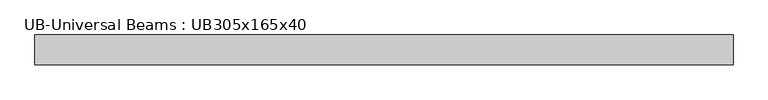
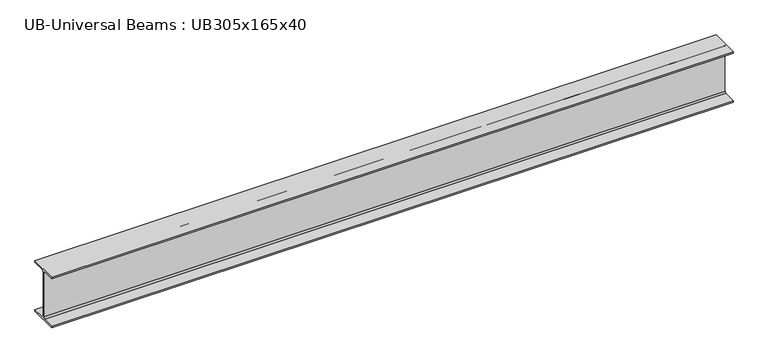
"""IFC4 building model written with IfcOpenShell, lengths in millimetres: beam geometry, UB-Universal Beams : UB305x165x40."""

from ifc_helpers import new_model, si_unit, point, frame, frame_2d, origin, place, context, project, spatial, polyline, circle_curve, trimmed, segment, composite_curve, outline, extrude, source, transform, mapped, element, save


def ub_universal_beams_ub305x165x40_f58164a9(model_context):
    return source(origin(), model_context, "Body", "SweptSolid", [
        extrude(outline(composite_curve([segment(polyline([(82.5, -141.5), (82.5, -151.7), (-82.5, -151.7), (-82.5, -141.5), (-11.9, -141.5)]), True, "CONTINUOUS"), segment(trimmed(circle_curve(frame_2d((-11.9, -132.6)), 8.9), [point((-11.9, -141.5))], [point((-3.0, -132.6))], True, "CARTESIAN"), True, "CONTINUOUS"), segment(polyline([(-3.0, -132.6), (-3.0, 132.6)]), True, "CONTINUOUS"), segment(trimmed(circle_curve(frame_2d((-11.9, 132.6)), 8.9), [point((-3.0, 132.6))], [point((-11.9, 141.5))], True, "CARTESIAN"), True, "CONTINUOUS"), segment(polyline([(-11.9, 141.5), (-82.5, 141.5), (-82.5, 151.7), (82.5, 151.7), (82.5, 141.5), (11.9, 141.5)]), True, "CONTINUOUS"), segment(trimmed(circle_curve(frame_2d((11.9, 132.6)), 8.9), [point((11.9, 141.5))], [point((3.0, 132.6))], True, "CARTESIAN"), True, "CONTINUOUS"), segment(polyline([(3.0, 132.6), (3.0, -132.6)]), True, "CONTINUOUS"), segment(trimmed(circle_curve(frame_2d((11.9, -132.6)), 8.9), [point((3.0, -132.6))], [point((11.9, -141.5))], True, "CARTESIAN"), True, "CONTINUOUS"), segment(polyline([(11.9, -141.5), (82.5, -141.5)]), True, "CONTINUOUS")], self_intersect=False)), frame((-1739.75, 0.0, 0.0), z_axis=(1.0, 0.0, 0.0), x_axis=(0.0, 1.0, 0.0)), (0.0, 0.0, 1.0), 3860.0),
    ])


if __name__ == "__main__":
    model = new_model("IFC4")
    model_context = context("Model", 3, world=origin())
    ifc_project = project(units=[si_unit("LENGTHUNIT", "METRE", prefix="MILLI")], contexts=[model_context])
    site = spatial("IfcSite", under=ifc_project)
    building = spatial("IfcBuilding", under=site)
    placement = place(None, origin())
    ub_universal_beams_ub305x165x40_shape = ub_universal_beams_ub305x165x40_f58164a9(model_context)
    element("IfcBeam", 1, ObjectType="UB-Universal Beams : UB305x165x40", at=placement, inside=building, context=model_context, shape_type="MappedRepresentation", body=[
        mapped(ub_universal_beams_ub305x165x40_shape, transform((0.0, 0.0, 0.0), x_axis=(1.0, 0.0, 0.0), y_axis=(0.0, 1.0, 0.0), z_axis=(0.0, 0.0, 1.0))),
    ])
    save(model, "model.ifc")

# Revit data of these elements
# Type "UB-Universal Beams : UB305x165x40"
#   Section Name Key = "UB305X165X40"
#   Width = 16.5 cm
#   Web Thickness = 0.6 cm
#   Web Fillet = 0.89 cm
#   Warping Constant = 164000.0 cm⁶
#   Torsional Moment of Inertia = 14.70 cm⁴
#   Section Area = 51.3 cm²
#   Plastic Modulus weak axis = 142.0 cm³
#   Plastic Modulus strong axis = 623.0 cm³
#   Nominal Weight = 40.2999 kgf/m
#   Moment of Inertia weak axis = 764.00 cm⁴
#   Moment of Inertia strong axis = 8503.00 cm⁴
#   Height = 30.34 cm
#   Flange Thickness = 1.02 cm
#   Elastic Modulus weak axis = 92.6 cm³
#   Elastic Modulus strong axis = 560.0 cm³
#   Centroid Vertical = 15.17 cm
#   Centroid Horizontal = 8.25 cm
#   Bolt Spacing = 9.0 cm
#   Length [instance default] = 1500 mm
#   Structural Material [instance default] = Metal - Steel 43-275
#   Type Comments = ""
#   Assembly Code = ""
# Element 1 (IfcBeam, "UB-Universal Beams : UB305x165x40")
#   Materials on its faces: "Metal - Steel 43-275"
# Materials
#   "Metal - Steel 43-275": class "Metal", colour RGB 247 247 247, transparency 0, Cost = 0
